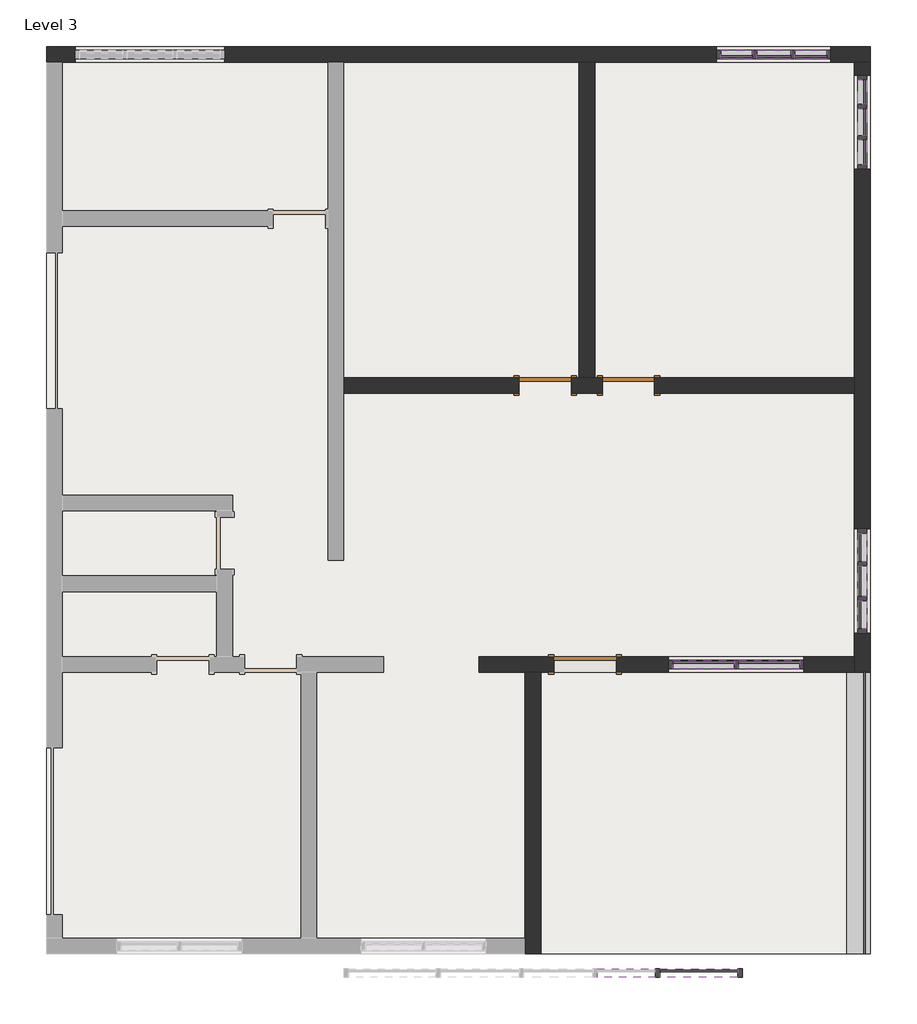
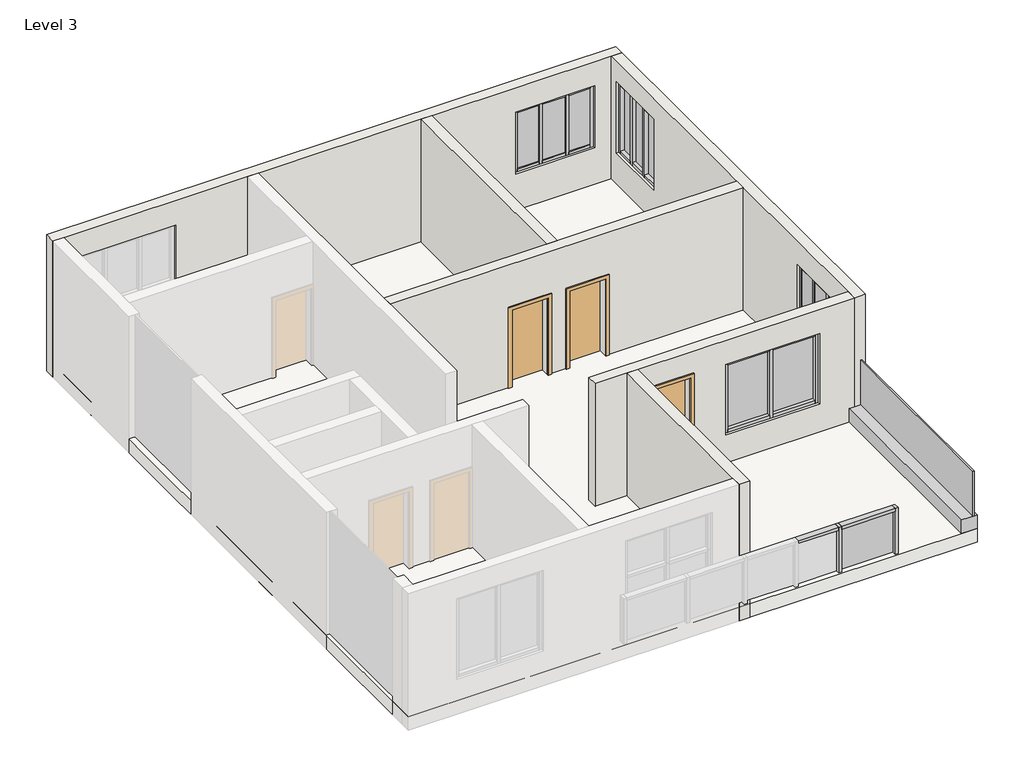
# One storey, part 2 of 2: 41 members, 13 plates, 6 walls, 3 doors, 1 proxy, 1 roof.
"""IFC4 building model written with IfcOpenShell, lengths in millimetres."""

from ifc_helpers import new_model, si_unit, frame, origin, place, context, project, spatial, polyline, outline, extrude, faceted_brep, transform, mapped, element, save
from components import generic_models_4_generic_models_4_fc34fd45, door_a1484949, door_85036156, door_a90ba1ad, member_f1f71bde, member_5535eeb3, member_2ebf4a73, member_dc106669, member_bc7dbe04, member_56906109, member_466b835c, member_843225dc, member_7096a90e, member_3005f220, member_87430b41, member_fcbfb253, member_1929af86, member_d9ff3611, member_6335abfa, member_1825c13a, member_d2e7e466, member_7dabcdc2, member_870cb0cc, system_panel_glazed_df399847, system_panel_glazed_d4ab74e0, system_panel_glazed_c2792dd2, system_panel_glazed_33c81725, system_panel_glazed_28e9ce38, system_panel_glazed_71b5d3b3, system_panel_glazed_2b1bd5bc, system_panel_glazed_349dd858, system_panel_glazed_9bdbffb3

model = new_model("IFC4")

# Units and contexts
model_context = context("Model", 3, world=origin())
ifc_project = project(units=[si_unit("LENGTHUNIT", "METRE", prefix="MILLI")], contexts=[model_context])

# Site, building, storey
site = spatial("IfcSite", under=ifc_project)
building = spatial("IfcBuilding", under=site)
storey = spatial("IfcBuildingStorey", under=building, Name="Level 3", Elevation=6096.0)

# Proxy
placement = place(None, origin())
generic_models_4_generic_models_4_shape = generic_models_4_generic_models_4_fc34fd45(model_context)
element("IfcBuildingElementProxy", 1, Name="Generic Models 4 : Generic Models 4", ObjectType="Generic Models 4 : Generic Models 4", at=placement, inside=storey, context=model_context, shape_type="MappedRepresentation", body=[
    mapped(generic_models_4_generic_models_4_shape, transform((0.0, 0.0, 0.0), x_axis=(1.0, 0.0, 0.0), y_axis=(0.0, 1.0, 0.0), z_axis=(0.0, 0.0, 1.0))),
])

# Doors
door_shape = door_a1484949(model_context)
element("IfcDoor", 2, ObjectType="Single-Flush : 30\" x 80\"", at=placement, inside=storey, context=model_context, shape_type="MappedRepresentation", body=[
    mapped(door_shape, transform((-12995.791855, -5548.3538163, 6096.0), x_axis=(1.0, 0.0, 0.0), y_axis=(0.0, 1.0, 0.0), z_axis=(0.0, 0.0, 1.0))),
])
door_2_shape = door_85036156(model_context)
element("IfcDoor", 3, ObjectType="Single-Flush : 30\" x 80\"", at=placement, inside=storey, context=model_context, shape_type="MappedRepresentation", body=[
    mapped(door_2_shape, transform((-11776.591855, -5548.3538163, 6096.0), x_axis=(-1.0, 0.0, 0.0), y_axis=(0.0, -1.0, 0.0), z_axis=(0.0, 0.0, 1.0))),
])
door_3_shape = door_a90ba1ad(model_context)
element("IfcDoor", 4, ObjectType="Single-Flush : 36\" x 84\"", at=placement, inside=storey, context=model_context, shape_type="MappedRepresentation", body=[
    mapped(door_3_shape, transform((-12411.591855, -9625.0538163, 6451.6), x_axis=(-1.0, 0.0, 0.0), y_axis=(0.0, -1.0, 0.0), z_axis=(0.0, 0.0, 1.0))),
])

# Members
member_shape = member_f1f71bde(model_context)
element("IfcMember", 5, ObjectType="Rectangular Mullion : 2.5\" x 5\" rectangular", at=placement, inside=storey, context=model_context, shape_type="MappedRepresentation", body=[
    mapped(member_shape, transform((-10233.541855, -9625.0538163, 8602.9452062), x_axis=(0.0, 0.0, 1.0), y_axis=(0.0, -1.0, 0.0), z_axis=(1.0, 0.0, 0.0))),
])
element("IfcMember", 6, ObjectType="Rectangular Mullion : 2.5\" x 5\" rectangular", at=placement, inside=storey, context=model_context, shape_type="MappedRepresentation", body=[
    mapped(member_shape, transform((-9274.691855, -9625.0538163, 8602.9452062), x_axis=(0.0, 0.0, 1.0), y_axis=(0.0, -1.0, 0.0), z_axis=(1.0, 0.0, 0.0))),
])
element("IfcMember", 7, ObjectType="Rectangular Mullion : 2.5\" x 5\" rectangular", at=placement, inside=storey, context=model_context, shape_type="MappedRepresentation", body=[
    mapped(member_shape, transform((-10170.041855, -9625.0538163, 7028.819863), x_axis=(0.0, 0.0, -1.0), y_axis=(0.0, -1.0, 0.0), z_axis=(-1.0, 0.0, 0.0))),
])
element("IfcMember", 8, ObjectType="Rectangular Mullion : 2.5\" x 5\" rectangular", at=placement, inside=storey, context=model_context, shape_type="MappedRepresentation", body=[
    mapped(member_shape, transform((-11128.891855, -9625.0538163, 7028.819863), x_axis=(0.0, 0.0, -1.0), y_axis=(0.0, -1.0, 0.0), z_axis=(-1.0, 0.0, 0.0))),
])
member_2_shape = member_5535eeb3(model_context)
element("IfcMember", 9, ObjectType="Rectangular Mullion : 2.5\" x 5\" rectangular", at=placement, inside=storey, context=model_context, shape_type="MappedRepresentation", body=[
    mapped(member_2_shape, transform((-9344.541855, -709.6538163, 8602.9452062), x_axis=(0.0, 0.0, 1.0), y_axis=(0.0, 1.0, 0.0), z_axis=(-1.0, 0.0, 0.0))),
])
element("IfcMember", 10, ObjectType="Rectangular Mullion : 2.5\" x 5\" rectangular", at=placement, inside=storey, context=model_context, shape_type="MappedRepresentation", body=[
    mapped(member_2_shape, transform((-10430.391855, -709.6538163, 8602.9452062), x_axis=(0.0, 0.0, 1.0), y_axis=(0.0, 1.0, 0.0), z_axis=(-1.0, 0.0, 0.0))),
])
member_3_shape = member_2ebf4a73(model_context)
element("IfcMember", 11, ObjectType="Rectangular Mullion : 2.5\" x 5\" rectangular", at=placement, inside=storey, context=model_context, shape_type="MappedRepresentation", body=[
    mapped(member_3_shape, transform((-9903.341855, -709.6538163, 8602.9452062), x_axis=(0.0, 0.0, 1.0), y_axis=(0.0, 1.0, 0.0), z_axis=(-1.0, 0.0, 0.0))),
])
element("IfcMember", 12, ObjectType="Rectangular Mullion : 2.5\" x 5\" rectangular", at=placement, inside=storey, context=model_context, shape_type="MappedRepresentation", body=[
    mapped(member_3_shape, transform((-9408.041855, -709.6538163, 7214.1130698), x_axis=(0.0, 0.0, -1.0), y_axis=(0.0, 1.0, 0.0), z_axis=(1.0, 0.0, 0.0))),
])
element("IfcMember", 13, ObjectType="Rectangular Mullion : 2.5\" x 5\" rectangular", at=placement, inside=storey, context=model_context, shape_type="MappedRepresentation", body=[
    mapped(member_2_shape, transform((-9966.841855, -709.6538163, 7214.1130698), x_axis=(0.0, 0.0, -1.0), y_axis=(0.0, 1.0, 0.0), z_axis=(1.0, 0.0, 0.0))),
])
element("IfcMember", 14, ObjectType="Rectangular Mullion : 2.5\" x 5\" rectangular", at=placement, inside=storey, context=model_context, shape_type="MappedRepresentation", body=[
    mapped(member_2_shape, transform((-8880.991855, -709.6538163, 7214.1130698), x_axis=(0.0, 0.0, -1.0), y_axis=(0.0, 1.0, 0.0), z_axis=(1.0, 0.0, 0.0))),
])
member_4_shape = member_dc106669(model_context)
element("IfcMember", 15, ObjectType="Rectangular Mullion : 2.5\" x 5\" rectangular", at=placement, inside=storey, context=model_context, shape_type="MappedRepresentation", body=[
    mapped(member_4_shape, transform((-8360.291855, -8691.6038163, 8612.8125833), x_axis=(0.0, 0.0, 1.0), y_axis=(1.0, 0.0, 0.0), z_axis=(0.0, 1.0, 0.0))),
])
element("IfcMember", 16, ObjectType="Rectangular Mullion : 2.5\" x 5\" rectangular", at=placement, inside=storey, context=model_context, shape_type="MappedRepresentation", body=[
    mapped(member_4_shape, transform((-8360.291855, -7707.3538163, 8612.8125833), x_axis=(0.0, 0.0, 1.0), y_axis=(1.0, 0.0, 0.0), z_axis=(0.0, 1.0, 0.0))),
])
member_5_shape = member_bc7dbe04(model_context)
element("IfcMember", 17, ObjectType="Rectangular Mullion : 2.5\" x 5\" rectangular", at=placement, inside=storey, context=model_context, shape_type="MappedRepresentation", body=[
    mapped(member_5_shape, transform((-8360.291855, -8183.6038163, 8612.8125833), x_axis=(0.0, 0.0, 1.0), y_axis=(1.0, 0.0, 0.0), z_axis=(0.0, 1.0, 0.0))),
])
member_6_shape = member_56906109(model_context)
element("IfcMember", 18, ObjectType="Rectangular Mullion : 2.5\" x 5\" rectangular", at=placement, inside=storey, context=model_context, shape_type="MappedRepresentation", body=[
    mapped(member_6_shape, transform((-8360.291855, -8151.8538163, 7118.0626114), x_axis=(0.0, 1.0, 0.0), y_axis=(1.0, 0.0, 0.0), z_axis=(0.0, 0.0, -1.0))),
])
element("IfcMember", 19, ObjectType="Rectangular Mullion : 2.5\" x 5\" rectangular", at=placement, inside=storey, context=model_context, shape_type="MappedRepresentation", body=[
    mapped(member_6_shape, transform((-8360.291855, -8659.8538163, 7118.0626114), x_axis=(0.0, 1.0, 0.0), y_axis=(1.0, 0.0, 0.0), z_axis=(0.0, 0.0, -1.0))),
])
element("IfcMember", 20, ObjectType="Rectangular Mullion : 2.5\" x 5\" rectangular", at=placement, inside=storey, context=model_context, shape_type="MappedRepresentation", body=[
    mapped(member_4_shape, transform((-8360.291855, -8120.1038163, 7118.0626114), x_axis=(0.0, 0.0, -1.0), y_axis=(1.0, 0.0, 0.0), z_axis=(0.0, -1.0, 0.0))),
])
element("IfcMember", 21, ObjectType="Rectangular Mullion : 2.5\" x 5\" rectangular", at=placement, inside=storey, context=model_context, shape_type="MappedRepresentation", body=[
    mapped(member_4_shape, transform((-8360.291855, -9104.3538163, 7118.0626114), x_axis=(0.0, 0.0, -1.0), y_axis=(1.0, 0.0, 0.0), z_axis=(0.0, -1.0, 0.0))),
])
element("IfcMember", 22, ObjectType="Rectangular Mullion : 2.5\" x 5\" rectangular", at=placement, inside=storey, context=model_context, shape_type="MappedRepresentation", body=[
    mapped(member_5_shape, transform((-8360.291855, -8628.1038163, 7118.0626114), x_axis=(0.0, 0.0, -1.0), y_axis=(1.0, 0.0, 0.0), z_axis=(0.0, -1.0, 0.0))),
])
member_7_shape = member_466b835c(model_context)
element("IfcMember", 23, ObjectType="Rectangular Mullion : 2.5\" x 5\" rectangular", at=placement, inside=storey, context=model_context, shape_type="MappedRepresentation", body=[
    mapped(member_7_shape, transform((-8360.291855, -7643.8538163, 7118.0626114), x_axis=(0.0, 1.0, 0.0), y_axis=(1.0, 0.0, 0.0), z_axis=(0.0, 0.0, -1.0))),
])
element("IfcMember", 24, ObjectType="Rectangular Mullion : 2.5\" x 5\" rectangular", at=placement, inside=storey, context=model_context, shape_type="MappedRepresentation", body=[
    mapped(member_7_shape, transform((-8360.291855, -9167.8538163, 8612.8125833), x_axis=(0.0, -1.0, 0.0), y_axis=(1.0, 0.0, 0.0), z_axis=(0.0, 0.0, 1.0))),
])
member_8_shape = member_843225dc(model_context)
element("IfcMember", 25, ObjectType="Rectangular Mullion : 2.5\" x 5\" rectangular", at=placement, inside=storey, context=model_context, shape_type="MappedRepresentation", body=[
    mapped(member_8_shape, transform((-8360.291855, -1439.9038163, 8687.804515), x_axis=(0.0, 0.0, 1.0), y_axis=(-1.0, 0.0, 0.0), z_axis=(0.0, -1.0, 0.0))),
])
element("IfcMember", 26, ObjectType="Rectangular Mullion : 2.5\" x 5\" rectangular", at=placement, inside=storey, context=model_context, shape_type="MappedRepresentation", body=[
    mapped(member_8_shape, transform((-8360.291855, -2322.5538163, 8687.804515), x_axis=(0.0, 0.0, 1.0), y_axis=(-1.0, 0.0, 0.0), z_axis=(0.0, -1.0, 0.0))),
])
member_9_shape = member_7096a90e(model_context)
element("IfcMember", 27, ObjectType="Rectangular Mullion : 2.5\" x 5\" rectangular", at=placement, inside=storey, context=model_context, shape_type="MappedRepresentation", body=[
    mapped(member_9_shape, transform((-8360.291855, -1897.1038163, 8687.804515), x_axis=(0.0, 0.0, 1.0), y_axis=(-1.0, 0.0, 0.0), z_axis=(0.0, -1.0, 0.0))),
])
member_10_shape = member_3005f220(model_context)
element("IfcMember", 28, ObjectType="Rectangular Mullion : 2.5\" x 5\" rectangular", at=placement, inside=storey, context=model_context, shape_type="MappedRepresentation", body=[
    mapped(member_10_shape, transform((-8360.291855, -1471.6538163, 7094.769598), x_axis=(0.0, -1.0, 0.0), y_axis=(-1.0, 0.0, 0.0), z_axis=(0.0, 0.0, -1.0))),
])
element("IfcMember", 29, ObjectType="Rectangular Mullion : 2.5\" x 5\" rectangular", at=placement, inside=storey, context=model_context, shape_type="MappedRepresentation", body=[
    mapped(member_10_shape, transform((-8360.291855, -1928.8538163, 7094.769598), x_axis=(0.0, -1.0, 0.0), y_axis=(-1.0, 0.0, 0.0), z_axis=(0.0, 0.0, -1.0))),
])
element("IfcMember", 30, ObjectType="Rectangular Mullion : 2.5\" x 5\" rectangular", at=placement, inside=storey, context=model_context, shape_type="MappedRepresentation", body=[
    mapped(member_9_shape, transform((-8360.291855, -1503.4038163, 7094.769598), x_axis=(0.0, 0.0, -1.0), y_axis=(-1.0, 0.0, 0.0), z_axis=(0.0, 1.0, 0.0))),
])
element("IfcMember", 31, ObjectType="Rectangular Mullion : 2.5\" x 5\" rectangular", at=placement, inside=storey, context=model_context, shape_type="MappedRepresentation", body=[
    mapped(member_8_shape, transform((-8360.291855, -1960.6038163, 7094.769598), x_axis=(0.0, 0.0, -1.0), y_axis=(-1.0, 0.0, 0.0), z_axis=(0.0, 1.0, 0.0))),
])
element("IfcMember", 32, ObjectType="Rectangular Mullion : 2.5\" x 5\" rectangular", at=placement, inside=storey, context=model_context, shape_type="MappedRepresentation", body=[
    mapped(member_8_shape, transform((-8360.291855, -1077.9538163, 7094.769598), x_axis=(0.0, 0.0, -1.0), y_axis=(-1.0, 0.0, 0.0), z_axis=(0.0, 1.0, 0.0))),
])
member_11_shape = member_87430b41(model_context)
element("IfcMember", 33, ObjectType="Rectangular Mullion : 2.5\" x 5\" rectangular", at=placement, inside=storey, context=model_context, shape_type="MappedRepresentation", body=[
    mapped(member_11_shape, transform((-8360.291855, -1014.4538163, 8687.804515), x_axis=(0.0, 1.0, 0.0), y_axis=(-1.0, 0.0, 0.0), z_axis=(0.0, 0.0, 1.0))),
])
element("IfcMember", 34, ObjectType="Rectangular Mullion : 2.5\" x 5\" rectangular", at=placement, inside=storey, context=model_context, shape_type="MappedRepresentation", body=[
    mapped(member_11_shape, transform((-8360.291855, -2386.0538163, 7094.769598), x_axis=(0.0, -1.0, 0.0), y_axis=(-1.0, 0.0, 0.0), z_axis=(0.0, 0.0, -1.0))),
])
member_12_shape = member_fcbfb253(model_context)
element("IfcMember", 35, ObjectType="Rectangular Mullion : 2.5\" x 5\" rectangular", at=placement, inside=storey, context=model_context, shape_type="MappedRepresentation", body=[
    mapped(member_12_shape, transform((-9935.091855, -709.6538163, 7214.1130698), x_axis=(-1.0, 0.0, 0.0), y_axis=(0.0, 1.0, 0.0), z_axis=(0.0, 0.0, -1.0))),
])
element("IfcMember", 36, ObjectType="Rectangular Mullion : 2.5\" x 5\" rectangular", at=placement, inside=storey, context=model_context, shape_type="MappedRepresentation", body=[
    mapped(member_12_shape, transform((-9376.291855, -709.6538163, 7214.1130698), x_axis=(-1.0, 0.0, 0.0), y_axis=(0.0, 1.0, 0.0), z_axis=(0.0, 0.0, -1.0))),
])
member_13_shape = member_1929af86(model_context)
element("IfcMember", 37, ObjectType="Rectangular Mullion : 2.5\" x 5\" rectangular", at=placement, inside=storey, context=model_context, shape_type="MappedRepresentation", body=[
    mapped(member_13_shape, transform((-8817.491855, -709.6538163, 8602.9452062), x_axis=(1.0, 0.0, 0.0), y_axis=(0.0, 1.0, 0.0), z_axis=(0.0, 0.0, 1.0))),
])
element("IfcMember", 38, ObjectType="Rectangular Mullion : 2.5\" x 5\" rectangular", at=placement, inside=storey, context=model_context, shape_type="MappedRepresentation", body=[
    mapped(member_13_shape, transform((-10493.891855, -709.6538163, 7214.1130698), x_axis=(-1.0, 0.0, 0.0), y_axis=(0.0, 1.0, 0.0), z_axis=(0.0, 0.0, -1.0))),
])
member_14_shape = member_d9ff3611(model_context)
element("IfcMember", 39, ObjectType="Rectangular Mullion : 2.5\" x 5\" rectangular", at=placement, inside=storey, context=model_context, shape_type="MappedRepresentation", body=[
    mapped(member_14_shape, transform((-10201.791855, -9625.0538163, 7028.819863), x_axis=(1.0, 0.0, 0.0), y_axis=(0.0, -1.0, 0.0), z_axis=(0.0, 0.0, -1.0))),
])
member_15_shape = member_6335abfa(model_context)
element("IfcMember", 40, ObjectType="Rectangular Mullion : 2.5\" x 5\" rectangular", at=placement, inside=storey, context=model_context, shape_type="MappedRepresentation", body=[
    mapped(member_15_shape, transform((-9211.191855, -9625.0538163, 7028.819863), x_axis=(1.0, 0.0, 0.0), y_axis=(0.0, -1.0, 0.0), z_axis=(0.0, 0.0, -1.0))),
])
element("IfcMember", 41, ObjectType="Rectangular Mullion : 2.5\" x 5\" rectangular", at=placement, inside=storey, context=model_context, shape_type="MappedRepresentation", body=[
    mapped(member_15_shape, transform((-11192.391855, -9625.0538163, 8602.9452062), x_axis=(-1.0, 0.0, 0.0), y_axis=(0.0, -1.0, 0.0), z_axis=(0.0, 0.0, 1.0))),
])
member_16_shape = member_1825c13a(model_context)
element("IfcMember", 42, ObjectType="Rectangular Mullion : 2.5\" x 5\" rectangular", at=placement, inside=storey, context=model_context, shape_type="MappedRepresentation", body=[
    mapped(member_16_shape, transform((-10179.1432214, -14133.5538163, 7725.553622), x_axis=(0.0, 0.0, 1.0), y_axis=(0.0, -1.0, 0.0), z_axis=(1.0, 0.0, 0.0))),
])
member_17_shape = member_d2e7e466(model_context)
element("IfcMember", 43, ObjectType="Rectangular Mullion : 2.5\" x 5\" rectangular", at=placement, inside=storey, context=model_context, shape_type="MappedRepresentation", body=[
    mapped(member_17_shape, transform((-11383.5265548, -14133.5538163, 7725.553622), x_axis=(0.0, 0.0, 1.0), y_axis=(0.0, -1.0, 0.0), z_axis=(1.0, 0.0, 0.0))),
])
member_18_shape = member_7dabcdc2(model_context)
element("IfcMember", 44, ObjectType="Rectangular Mullion : 2.5\" x 5\" rectangular", at=placement, inside=storey, context=model_context, shape_type="MappedRepresentation", body=[
    mapped(member_18_shape, transform((-11351.7765548, -14133.5538163, 6705.6), x_axis=(1.0, 0.0, 0.0), y_axis=(0.0, -1.0, 0.0), z_axis=(0.0, 0.0, -1.0))),
])
member_19_shape = member_870cb0cc(model_context)
element("IfcMember", 45, ObjectType="Rectangular Mullion : 2.5\" x 5\" rectangular", at=placement, inside=storey, context=model_context, shape_type="MappedRepresentation", body=[
    mapped(member_19_shape, transform((-10115.6432214, -14133.5538163, 6705.6), x_axis=(1.0, 0.0, 0.0), y_axis=(0.0, -1.0, 0.0), z_axis=(0.0, 0.0, -1.0))),
])

# Plates
system_panel_glazed_shape = system_panel_glazed_df399847(model_context)
element("IfcPlate", 46, ObjectType="System Panel : Glazed", at=placement, inside=storey, context=model_context, shape_type="MappedRepresentation", body=[
    mapped(system_panel_glazed_shape, transform((-8360.291855, -8897.9788163, 7181.5626114), x_axis=(0.0, 1.0, 0.0), y_axis=(-1.0, 0.0, 0.0), z_axis=(0.0, 0.0, 1.0))),
])
element("IfcPlate", 47, ObjectType="System Panel : Glazed", at=placement, inside=storey, context=model_context, shape_type="MappedRepresentation", body=[
    mapped(system_panel_glazed_shape, transform((-8360.291855, -7913.7288163, 7181.5626114), x_axis=(0.0, 1.0, 0.0), y_axis=(-1.0, 0.0, 0.0), z_axis=(0.0, 0.0, 1.0))),
])
system_panel_glazed_2_shape = system_panel_glazed_d4ab74e0(model_context)
element("IfcPlate", 48, ObjectType="System Panel : Glazed", at=placement, inside=storey, context=model_context, shape_type="MappedRepresentation", body=[
    mapped(system_panel_glazed_2_shape, transform((-8360.291855, -8405.8538163, 7181.5626114), x_axis=(0.0, 1.0, 0.0), y_axis=(-1.0, 0.0, 0.0), z_axis=(0.0, 0.0, 1.0))),
])
system_panel_glazed_3_shape = system_panel_glazed_c2792dd2(model_context)
element("IfcPlate", 49, ObjectType="System Panel : Glazed", at=placement, inside=storey, context=model_context, shape_type="MappedRepresentation", body=[
    mapped(system_panel_glazed_3_shape, transform((-8360.291855, -1258.9288163, 7158.269598), x_axis=(0.0, -1.0, 0.0), y_axis=(1.0, 0.0, 0.0), z_axis=(0.0, 0.0, 1.0))),
])
element("IfcPlate", 50, ObjectType="System Panel : Glazed", at=placement, inside=storey, context=model_context, shape_type="MappedRepresentation", body=[
    mapped(system_panel_glazed_3_shape, transform((-8360.291855, -2141.5788163, 7158.269598), x_axis=(0.0, -1.0, 0.0), y_axis=(1.0, 0.0, 0.0), z_axis=(0.0, 0.0, 1.0))),
])
system_panel_glazed_4_shape = system_panel_glazed_33c81725(model_context)
element("IfcPlate", 51, ObjectType="System Panel : Glazed", at=placement, inside=storey, context=model_context, shape_type="MappedRepresentation", body=[
    mapped(system_panel_glazed_4_shape, transform((-8360.291855, -1700.2538163, 7158.269598), x_axis=(0.0, -1.0, 0.0), y_axis=(1.0, 0.0, 0.0), z_axis=(0.0, 0.0, 1.0))),
])
system_panel_glazed_5_shape = system_panel_glazed_28e9ce38(model_context)
element("IfcPlate", 52, ObjectType="System Panel : Glazed", at=placement, inside=storey, context=model_context, shape_type="MappedRepresentation", body=[
    mapped(system_panel_glazed_5_shape, transform((-9112.766855, -709.6538163, 7277.6130698), x_axis=(-1.0, 0.0, 0.0), y_axis=(0.0, -1.0, 0.0), z_axis=(0.0, 0.0, 1.0))),
])
element("IfcPlate", 53, ObjectType="System Panel : Glazed", at=placement, inside=storey, context=model_context, shape_type="MappedRepresentation", body=[
    mapped(system_panel_glazed_5_shape, transform((-10198.616855, -709.6538163, 7277.6130698), x_axis=(-1.0, 0.0, 0.0), y_axis=(0.0, -1.0, 0.0), z_axis=(0.0, 0.0, 1.0))),
])
system_panel_glazed_6_shape = system_panel_glazed_71b5d3b3(model_context)
element("IfcPlate", 54, ObjectType="System Panel : Glazed", at=placement, inside=storey, context=model_context, shape_type="MappedRepresentation", body=[
    mapped(system_panel_glazed_6_shape, transform((-9655.691855, -709.6538163, 7277.6130698), x_axis=(-1.0, 0.0, 0.0), y_axis=(0.0, -1.0, 0.0), z_axis=(0.0, 0.0, 1.0))),
])
system_panel_glazed_7_shape = system_panel_glazed_2b1bd5bc(model_context)
element("IfcPlate", 55, ObjectType="System Panel : Glazed", at=placement, inside=storey, context=model_context, shape_type="MappedRepresentation", body=[
    mapped(system_panel_glazed_7_shape, transform((-10681.216855, -9625.0538163, 7092.319863), x_axis=(1.0, 0.0, 0.0), y_axis=(0.0, 1.0, 0.0), z_axis=(0.0, 0.0, 1.0))),
])
element("IfcPlate", 56, ObjectType="System Panel : Glazed", at=placement, inside=storey, context=model_context, shape_type="MappedRepresentation", body=[
    mapped(system_panel_glazed_7_shape, transform((-9722.366855, -9625.0538163, 7092.319863), x_axis=(1.0, 0.0, 0.0), y_axis=(0.0, 1.0, 0.0), z_axis=(0.0, 0.0, 1.0))),
])
system_panel_glazed_8_shape = system_panel_glazed_349dd858(model_context)
element("IfcPlate", 57, ObjectType="System Panel : Glazed", at=placement, inside=storey, context=model_context, shape_type="MappedRepresentation", body=[
    mapped(system_panel_glazed_8_shape, transform((-8296.791855, -11796.7538163, 6705.6), x_axis=(0.0, 1.0, 0.0), y_axis=(-1.0, 0.0, 0.0), z_axis=(0.0, 0.0, 1.0))),
])
system_panel_glazed_9_shape = system_panel_glazed_9bdbffb3(model_context)
element("IfcPlate", 58, ObjectType="System Panel : Glazed", at=placement, inside=storey, context=model_context, shape_type="MappedRepresentation", body=[
    mapped(system_panel_glazed_9_shape, transform((-10749.5848881, -14133.5538163, 6705.6), x_axis=(1.0, 0.0, 0.0), y_axis=(0.0, 1.0, 0.0), z_axis=(0.0, 0.0, 1.0))),
])

# Roof
element("IfcRoof", 59, ObjectType="Generic - 12\"", at=placement, inside=storey, context=model_context, shape_type="SweptSolid", body=[
    extrude(outline(polyline([(-20285.591855, -595.3538163), (-8245.991855, -595.3538163), (-8245.991855, -13854.1538163), (-20285.591855, -13854.1538163), (-20285.591855, -595.3538163)])), frame((0.0, 0.0, 6096.0), z_axis=(0.0, 0.0, 1.0), x_axis=(1.0, 0.0, 0.0)), (0.0, 0.0, 1.0), 304.8),
])

# Walls
element("IfcWall", 60, ObjectType="9\"", at=placement, inside=storey, context=model_context, shape_type="Brep", body=[
    faceted_brep([(-20285.591855, -823.9538163, 6096.0), (-20056.991855, -823.9538163, 6096.0), (-16170.791855, -823.9538163, 6096.0), (-15942.191855, -823.9538163, 6096.0), (-12500.491855, -823.9538163, 6096.0), (-12271.891855, -823.9538163, 6096.0), (-8474.591855, -823.9538163, 6096.0), (-8245.991855, -823.9538163, 6096.0), (-8245.991855, -823.9538163, 9144.0), (-8474.591855, -823.9538163, 9144.0), (-12271.891855, -823.9538163, 9144.0), (-12500.491855, -823.9538163, 9144.0), (-15942.191855, -823.9538163, 9144.0), (-16170.791855, -823.9538163, 9144.0), (-20056.991855, -823.9538163, 9144.0), (-20285.591855, -823.9538163, 9144.0), (-8817.491855, -823.9538163, 8602.9452062), (-8817.491855, -823.9538163, 7214.1130698), (-10493.891855, -823.9538163, 7214.1130698), (-10493.891855, -823.9538163, 8602.9452062), (-19866.491855, -823.9538163, 7292.9915007), (-19866.491855, -823.9538163, 8591.2496538), (-17682.091855, -823.9538163, 8591.2496538), (-17682.091855, -823.9538163, 7292.9915007), (-8245.991855, -595.3538163, 6096.0), (-20285.591855, -595.3538163, 6096.0), (-20285.591855, -595.3538163, 9144.0), (-8245.991855, -595.3538163, 9144.0), (-8817.491855, -595.3538163, 7214.1130698), (-8817.491855, -595.3538163, 8602.9452062), (-10493.891855, -595.3538163, 8602.9452062), (-10493.891855, -595.3538163, 7214.1130698), (-19866.491855, -595.3538163, 8591.2496538), (-19866.491855, -595.3538163, 7292.9915007), (-17682.091855, -595.3538163, 7292.9915007), (-17682.091855, -595.3538163, 8591.2496538)], [[[0, 1, 2, 3, 4, 5, 6, 7, 8, 9, 10, 11, 12, 13, 14, 15], [16, 17, 18, 19], [20, 21, 22, 23]], [[24, 25, 26, 27], [28, 29, 30, 31], [32, 33, 34, 35]], [[7, 6, 5, 4, 3, 2, 1, 0, 25, 24]], [[15, 14, 13, 12, 11, 10, 9, 8, 27, 26]], [[8, 7, 24, 27]], [[0, 15, 26, 25]], [[28, 17, 16, 29]], [[29, 16, 19, 30]], [[30, 19, 18, 31]], [[17, 28, 31, 18]], [[32, 21, 20, 33]], [[21, 32, 35, 22]], [[22, 35, 34, 23]], [[33, 20, 23, 34]]]),
])
element("IfcWall", 61, ObjectType="9\"", at=placement, inside=storey, context=model_context, shape_type="Brep", body=[
    faceted_brep([(-8474.591855, -823.9538163, 6096.0), (-8474.591855, -5434.0538163, 6096.0), (-8474.591855, -5662.6538163, 6096.0), (-8474.591855, -9510.7538163, 6096.0), (-8474.591855, -9739.3538163, 6096.0), (-8474.591855, -9739.3538163, 9144.0), (-8474.591855, -9510.7538163, 9144.0), (-8474.591855, -5662.6538163, 9144.0), (-8474.591855, -5434.0538163, 9144.0), (-8474.591855, -823.9538163, 9144.0), (-8474.591855, -9167.8538163, 8612.8125833), (-8474.591855, -9167.8538163, 7118.0626114), (-8474.591855, -7643.8538163, 7118.0626114), (-8474.591855, -7643.8538163, 8612.8125833), (-8474.591855, -1014.4538163, 7094.769598), (-8474.591855, -1014.4538163, 8687.804515), (-8474.591855, -2386.0538163, 8687.804515), (-8474.591855, -2386.0538163, 7094.769598), (-8245.991855, -9739.3538163, 6096.0), (-8245.991855, -823.9538163, 6096.0), (-8245.991855, -823.9538163, 9144.0), (-8245.991855, -9739.3538163, 9144.0), (-8245.991855, -9167.8538163, 7118.0626114), (-8245.991855, -9167.8538163, 8612.8125833), (-8245.991855, -7643.8538163, 8612.8125833), (-8245.991855, -7643.8538163, 7118.0626114), (-8245.991855, -1014.4538163, 8687.804515), (-8245.991855, -1014.4538163, 7094.769598), (-8245.991855, -2386.0538163, 7094.769598), (-8245.991855, -2386.0538163, 8687.804515)], [[[0, 1, 2, 3, 4, 5, 6, 7, 8, 9], [10, 11, 12, 13], [14, 15, 16, 17]], [[18, 19, 20, 21], [22, 23, 24, 25], [26, 27, 28, 29]], [[4, 3, 2, 1, 0, 19, 18]], [[9, 8, 7, 6, 5, 21, 20]], [[0, 9, 20, 19]], [[5, 4, 18, 21]], [[10, 23, 22, 11]], [[23, 10, 13, 24]], [[24, 13, 12, 25]], [[11, 22, 25, 12]], [[14, 27, 26, 15]], [[15, 26, 29, 16]], [[16, 29, 28, 17]], [[27, 14, 17, 28]]]),
])
element("IfcWall", 62, ObjectType="9\"", at=placement, inside=storey, context=model_context, shape_type="Brep", body=[
    faceted_brep([(-8474.591855, -9510.7538163, 6096.0), (-13960.991855, -9510.7538163, 6096.0), (-13960.991855, -9510.7538163, 9144.0), (-8474.591855, -9510.7538163, 9144.0), (-12868.791855, -9510.7538163, 6451.6), (-11954.391855, -9510.7538163, 6451.6), (-11954.391855, -9510.7538163, 8585.2), (-12868.791855, -9510.7538163, 8585.2), (-11192.391855, -9510.7538163, 8602.9452062), (-11192.391855, -9510.7538163, 7028.819863), (-9211.191855, -9510.7538163, 7028.819863), (-9211.191855, -9510.7538163, 8602.9452062), (-13960.991855, -9739.3538163, 6096.0), (-13287.891855, -9739.3538163, 6096.0), (-13059.291855, -9739.3538163, 6096.0), (-8474.591855, -9739.3538163, 6096.0), (-8474.591855, -9739.3538163, 9144.0), (-13059.291855, -9739.3538163, 9144.0), (-13287.891855, -9739.3538163, 9144.0), (-13960.991855, -9739.3538163, 9144.0), (-11954.391855, -9739.3538163, 6451.6), (-12868.791855, -9739.3538163, 6451.6), (-12868.791855, -9739.3538163, 8585.2), (-11954.391855, -9739.3538163, 8585.2), (-11192.391855, -9739.3538163, 7028.819863), (-11192.391855, -9739.3538163, 8602.9452062), (-9211.191855, -9739.3538163, 8602.9452062), (-9211.191855, -9739.3538163, 7028.819863)], [[[0, 1, 2, 3], [4, 5, 6, 7], [8, 9, 10, 11]], [[12, 13, 14, 15, 16, 17, 18, 19], [20, 21, 22, 23], [24, 25, 26, 27]], [[1, 0, 15, 14, 13, 12]], [[2, 1, 12, 19]], [[3, 2, 19, 18, 17, 16]], [[0, 3, 16, 15]], [[21, 20, 5, 4]], [[22, 21, 4, 7]], [[23, 22, 7, 6]], [[20, 23, 6, 5]], [[24, 9, 8, 25]], [[25, 8, 11, 26]], [[26, 11, 10, 27]], [[9, 24, 27, 10]]]),
])
element("IfcWall", 63, ObjectType="9\"", at=placement, inside=storey, context=model_context, shape_type="Brep", body=[
    faceted_brep([(-13287.891855, -9739.3538163, 6096.0), (-13287.891855, -13625.5538163, 6096.0), (-13287.891855, -13854.1538163, 6096.0), (-13287.891855, -13854.1538163, 9144.0), (-13287.891855, -13625.5538163, 9144.0), (-13287.891855, -9739.3538163, 9144.0), (-13059.291855, -9739.3538163, 6096.0), (-13059.291855, -9739.3538163, 9144.0), (-13059.291855, -13854.1538163, 9144.0), (-13059.291855, -13854.1538163, 6096.0)], [[[0, 1, 2, 3, 4, 5]], [[6, 7, 8, 9]], [[2, 1, 0, 6, 9]], [[5, 4, 3, 8, 7]], [[0, 5, 7, 6]], [[3, 2, 9, 8]]]),
])
element("IfcWall", 64, ObjectType="9\"", at=placement, inside=storey, context=model_context, shape_type="Brep", body=[
    faceted_brep([(-12614.791855, -5662.6538163, 6096.0), (-12157.591855, -5662.6538163, 6096.0), (-12157.591855, -5662.6538163, 8128.0), (-11395.591855, -5662.6538163, 8128.0), (-11395.591855, -5662.6538163, 6096.0), (-8474.591855, -5662.6538163, 6096.0), (-8474.591855, -5662.6538163, 9144.0), (-15942.191855, -5662.6538163, 9144.0), (-15942.191855, -5662.6538163, 6096.0), (-13376.791855, -5662.6538163, 6096.0), (-13376.791855, -5662.6538163, 8128.0), (-12614.791855, -5662.6538163, 8128.0), (-12157.591855, -5434.0538163, 8128.0), (-12157.591855, -5434.0538163, 6096.0), (-12271.891855, -5434.0538163, 6096.0), (-12500.491855, -5434.0538163, 6096.0), (-12614.791855, -5434.0538163, 6096.0), (-12614.791855, -5434.0538163, 8128.0), (-13376.791855, -5434.0538163, 8128.0), (-13376.791855, -5434.0538163, 6096.0), (-15942.191855, -5434.0538163, 6096.0), (-15942.191855, -5434.0538163, 9144.0), (-12500.491855, -5434.0538163, 9144.0), (-12271.891855, -5434.0538163, 9144.0), (-8474.591855, -5434.0538163, 9144.0), (-8474.591855, -5434.0538163, 6096.0), (-11395.591855, -5434.0538163, 6096.0), (-11395.591855, -5434.0538163, 8128.0)], [[[0, 1, 2, 3, 4, 5, 6, 7, 8, 9, 10, 11]], [[12, 13, 14, 15, 16, 17, 18, 19, 20, 21, 22, 23, 24, 25, 26, 27]], [[9, 8, 20, 19]], [[26, 25, 5, 4]], [[16, 15, 14, 13, 1, 0]], [[7, 6, 24, 23, 22, 21]], [[6, 5, 25, 24]], [[8, 7, 21, 20]], [[17, 16, 0, 11]], [[18, 17, 11, 10]], [[19, 18, 10, 9]], [[2, 1, 13, 12]], [[3, 2, 12, 27]], [[4, 3, 27, 26]]]),
])
element("IfcWall", 65, ObjectType="9\"", at=placement, inside=storey, context=model_context, shape_type="SweptSolid", body=[
    extrude(outline(polyline([(-12500.491855, -5434.0538163), (-12500.491855, -823.9538163), (-12271.891855, -823.9538163), (-12271.891855, -5434.0538163), (-12500.491855, -5434.0538163)])), frame((0.0, 0.0, 6096.0), z_axis=(0.0, 0.0, 1.0), x_axis=(1.0, 0.0, 0.0)), (0.0, 0.0, 1.0), 3048.0),
])

save(model, "model.ifc")

# Revit data of these elements
# Type "Single-Flush : 30\" x 80\""
#   Type Mark = "5"
#   Construction Type Id = "MDOOR"
#   Assembly Code = "C1020"
#   Analytic Construction = "Metal"
#   Thickness = 0' - 2"
#   Heat Transfer Coefficient (U) = 0.651978 BTU/(h·ft²·°F)
#   Height = 6' - 8"
#   Trim Projection Ext = 0' - 1"
#   Trim Projection Int = 0' - 1"
#   Trim Width = 0' - 3"
#   Width = 2' - 6"
#   Define Thermal Properties by = 1
#   Define Thermal Properties by = 1
#   Door Material = Door - Panel
#   Frame Material = Door - Frame
#   Visual Light Transmittance = 0
#   Solar Heat Gain Coefficient = 0
#   Function = (empty or 0)
#   Wall Closure = (empty or 0)
# Type "Single-Flush : 36\" x 84\""
#   Type Mark = "1"
#   Construction Type Id = "MDOOR"
#   Assembly Code = "C1020"
#   Analytic Construction = "Metal"
#   Thickness = 0' - 2"
#   Heat Transfer Coefficient (U) = 0.651978 BTU/(h·ft²·°F)
#   Height = 7' - 0"
#   Trim Projection Ext = 0' - 1"
#   Trim Projection Int = 0' - 1"
#   Trim Width = 0' - 3"
#   Width = 3' - 0"
#   Define Thermal Properties by = 1
#   Define Thermal Properties by = 1
#   Door Material = Door - Panel
#   Frame Material = Door - Frame
#   Visual Light Transmittance = 0
#   Solar Heat Gain Coefficient = 0
#   Function = (empty or 0)
#   Wall Closure = (empty or 0)
# Type "Rectangular Mullion : 2.5\" x 5\" rectangular"
#   built-in parameter 1007304 = 0.416667 (stored number, unit not read)
#   built-in parameter 1007301 = 0.104167 (stored number, unit not read)
#   built-in parameter 1007300 = 0.104167 (stored number, unit not read)
# Type "System Panel : Glazed"
#   Construction Type Id = "GSP4R"
#   Analytic Construction = "1/8 in Pilkington single glazing"
#   Visual Light Transmittance = 0.9
#   Solar Heat Gain Coefficient = 0.86
#   Heat Transfer Coefficient (U) = 1.18115 BTU/(h·ft²·°F)
#   Define Thermal Properties by = 1
# Type "Generic - 12\""
#   Assembly Code = "B1020"
#   Layers, outside or top first: 1' - 0" no material (function 1)
# Type "9\""
#   Assembly Code = "B2010"
#   Layers, outside or top first: 0' - 9" no material (function 1)
# Element 1 (IfcBuildingElementProxy, "Generic Models 4 : Generic Models 4")
#   Phase Created = New Construction
# Elements 2, 3 (IfcDoor, "Single-Flush : 30\" x 80\"")
#   Phase Created = New Construction
#   Materials on its faces: "Door - Frame", "Door - Panel"
# Element 4 (IfcDoor, "Single-Flush : 36\" x 84\"")
#   Phase Created = New Construction
#   Materials on its faces: "Door - Frame", "Door - Panel"
# Elements 5, 6, 7, 8, 9, 10, 11, 12, 13, 14, 15, 16, 17, 18, 19, 20, 21, 22, 23, 24, 25, 26, 27, 28, 29, 30, 31, 32, 33, 34, 35, 36, 37, 38, 39, 40, 41, 42, 43, 44, 45 (IfcMember, "Rectangular Mullion : 2.5\" x 5\" rectangular")
#   Phase Created = New Construction
#   Materials on its faces: "Aluminum"
# Elements 46, 47, 48, 49, 50, 51, 52, 53, 54, 55, 56, 57, 58 (IfcPlate, "System Panel : Glazed")
#   Phase Created = New Construction
#   Materials on its faces: "Glass"
# Element 59 (IfcRoof, "Generic - 12\"")
#   built-in parameter 1001705 = 21 (stored number, unit not read)
#   built-in parameter 1001710 = 33615
#   Phase Created = New Construction
#   Materials on its faces: "Default Roof"
# Elements 60, 61, 62, 63, 64, 65 (IfcWall, "9\"")
#   Top Offset = 0' - 0"
#   Base Offset = 0' - 0"
#   Unconnected Height = 10' - 0"
#   wall height = 10' - 0"
#   Phase Created = New Construction
#   Base Constraint = Level 3
#   Materials on its faces: "Default Wall"
# Materials
#   "Door - Panel": class "Wood", colour RGB 210 159 95, transparency 0, Cost = 0
#   "Door - Frame": colour RGB 118 70 51, transparency 0, Cost = 0
#   "Aluminum": class "Metal", colour RGB 247 247 247, transparency 0, Description = "Aluminum 6061", Cost = 0
#   "Glass": class "Glass", colour RGB 0 128 192, transparency 0.75, Description = "Soda Lime Glass", Cost = 0
#   "Default Roof": colour RGB 88 101 114, transparency 0, Cost = 0
#   "Default Wall": colour RGB 128 128 128, transparency 0, Cost = 0
